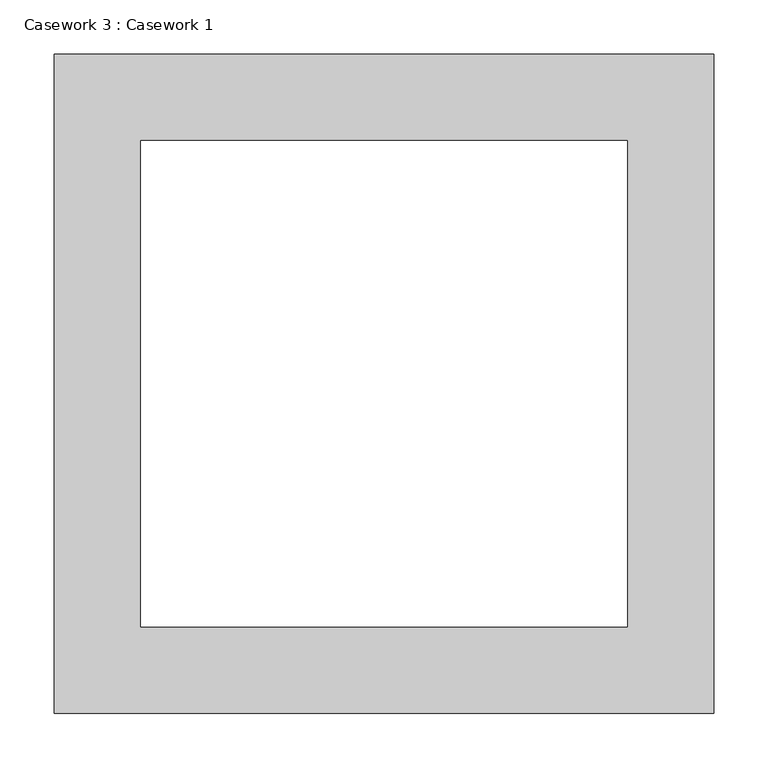
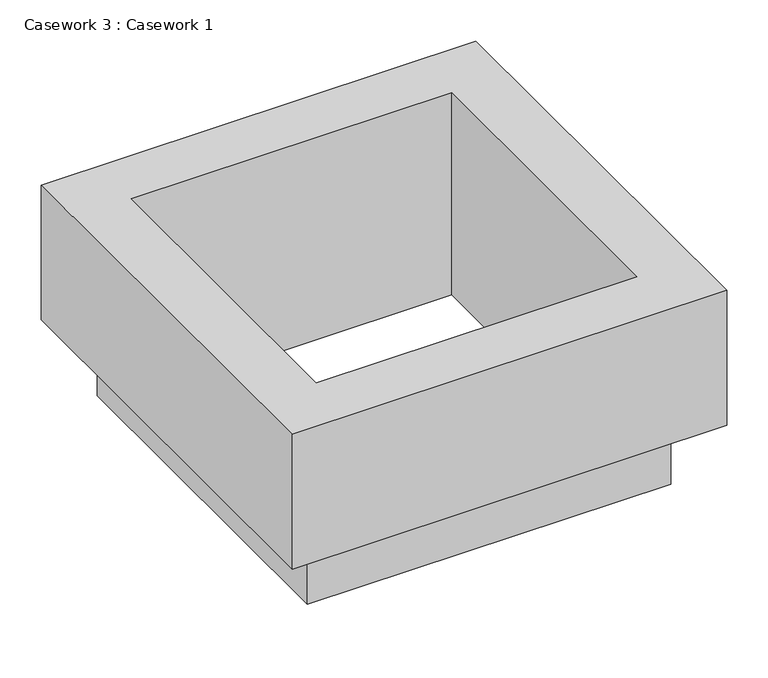
"""IFC4 building model written with IfcOpenShell, lengths in millimetres: furniture geometry, Casework 3 : Casework 1."""

from ifc_helpers import new_model, si_unit, origin, place, context, project, spatial, faceted_brep, source, transform, mapped, element, save


def casework_3_casework_1_4875a9a3(model_context):
    return source(origin(), model_context, "Body", "Brep", [
        faceted_brep([(-2011.9096214, -14053.8952964, 3550.0), (-2011.9096214, -14053.8952964, 3450.0), (-1501.9096214, -14053.8952964, 3450.0), (-1501.9096214, -14053.8952964, 3550.0), (-2061.9096214, -14103.8952964, 3750.0), (-2061.9096214, -14103.8952964, 3550.0), (-1451.9096214, -14103.8952964, 3550.0), (-1451.9096214, -14103.8952964, 3750.0), (-1981.9096214, -14023.8952964, 3450.0), (-1981.9096214, -14023.8952964, 3750.0), (-1531.9096214, -14023.8952964, 3750.0), (-1531.9096214, -14023.8952964, 3450.0), (-1501.9096214, -13543.8952964, 3450.0), (-1501.9096214, -13543.8952964, 3550.0), (-1451.9096214, -13493.8952964, 3550.0), (-1451.9096214, -13493.8952964, 3750.0), (-1531.9096214, -13573.8952964, 3750.0), (-1531.9096214, -13573.8952964, 3450.0), (-2011.9096214, -13543.8952964, 3450.0), (-2011.9096214, -13543.8952964, 3550.0), (-2061.9096214, -13493.8952964, 3550.0), (-2061.9096214, -13493.8952964, 3750.0), (-1981.9096214, -13573.8952964, 3750.0), (-1981.9096214, -13573.8952964, 3450.0)], [[[0, 1, 2, 3]], [[4, 5, 6, 7]], [[8, 9, 10, 11]], [[3, 2, 12, 13]], [[7, 6, 14, 15]], [[11, 10, 16, 17]], [[13, 12, 18, 19]], [[15, 14, 20, 21]], [[17, 16, 22, 23]], [[19, 18, 1, 0]], [[5, 20, 14, 6], [3, 13, 19, 0]], [[21, 20, 5, 4]], [[7, 15, 21, 4], [9, 22, 16, 10]], [[23, 22, 9, 8]], [[1, 18, 12, 2], [11, 17, 23, 8]]]),
    ])


if __name__ == "__main__":
    model = new_model("IFC4")
    model_context = context("Model", 3, world=origin())
    ifc_project = project(units=[si_unit("LENGTHUNIT", "METRE", prefix="MILLI")], contexts=[model_context])
    site = spatial("IfcSite", under=ifc_project)
    building = spatial("IfcBuilding", under=site)
    placement = place(None, origin())
    casework_3_casework_1_shape = casework_3_casework_1_4875a9a3(model_context)
    element("IfcFurniture", 1, ObjectType="Casework 3 : Casework 1", at=placement, inside=building, context=model_context, shape_type="MappedRepresentation", body=[
        mapped(casework_3_casework_1_shape, transform((0.0, 0.0, 0.0), x_axis=(1.0, 0.0, 0.0), y_axis=(0.0, 1.0, 0.0), z_axis=(0.0, 0.0, 1.0))),
    ])
    save(model, "model.ifc")
